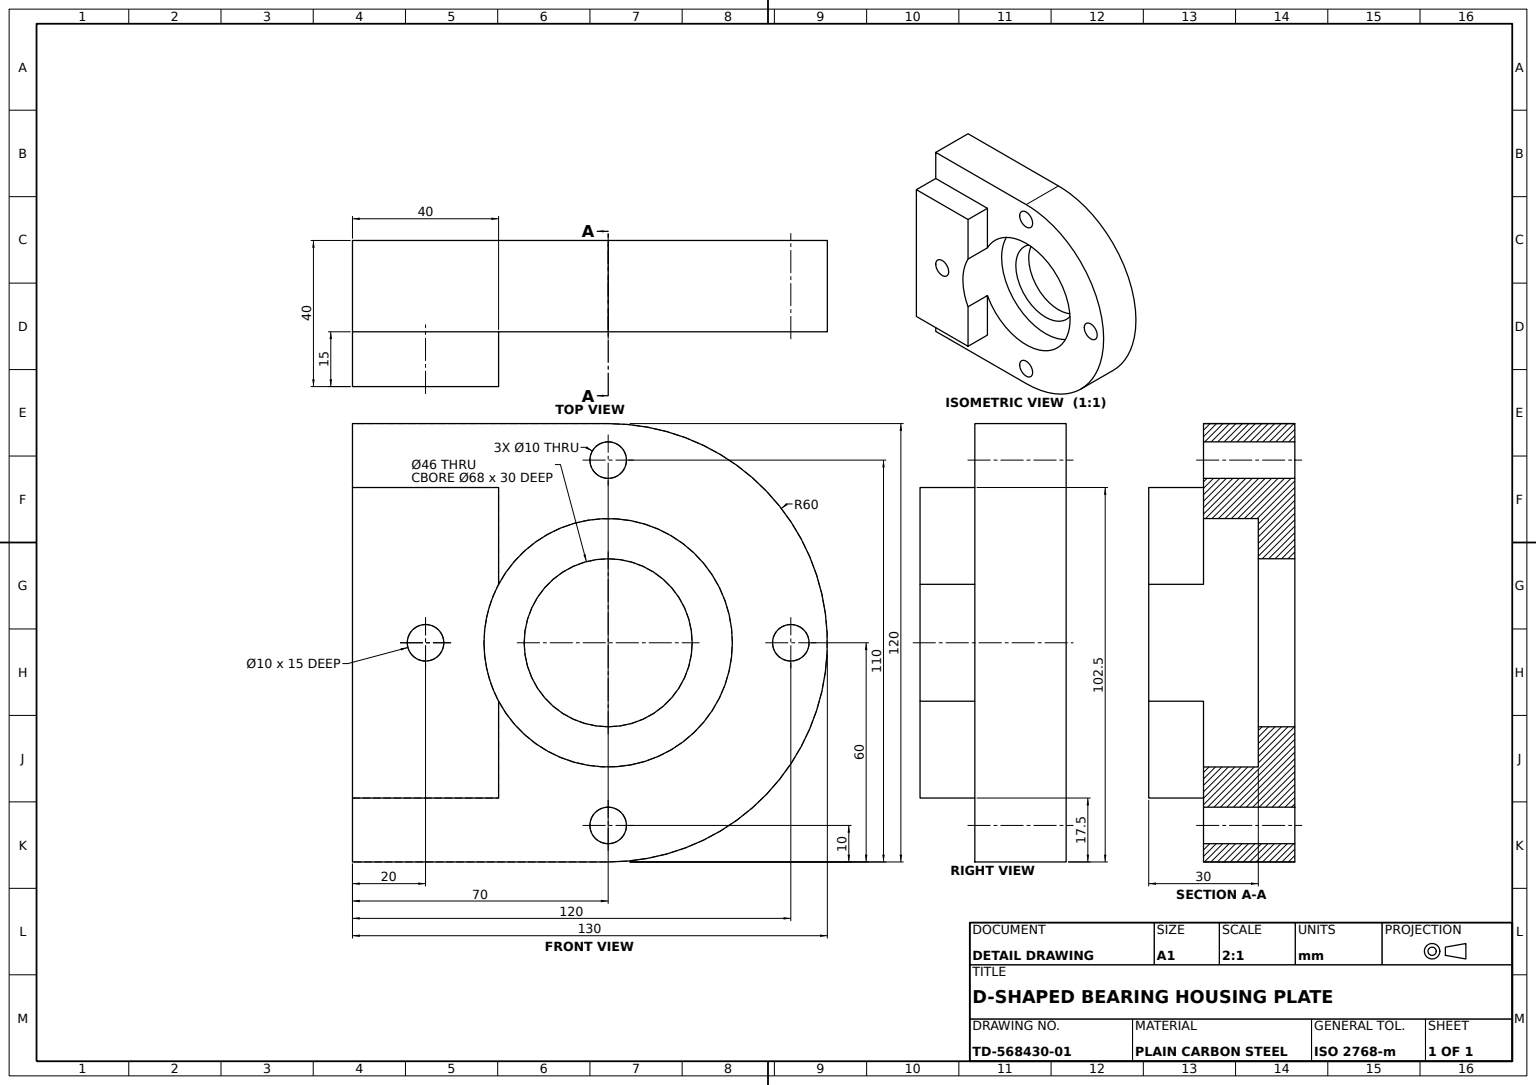
SolidWorks part; units mm, degrees
material "Plain Carbon Steel"
ref_plane "Front Plane" through (0, 0, 0) normal (0, 0, 1) x (1, 0, 0)
ref_plane "Top Plane" through (0, 0, 0) normal (0, 1, 0) x (1, 0, 0)
ref_plane "Right Plane" through (0, 0, 0) normal (1, 0, 0) x (0, 0, -1)
sketch "Base Plate Sketch" plane through (0, 0, 0) normal (0, 0, 1) x (1, 0, 0)
  line L0 (0, 0) -> (70, 0)
  line L2 (70, 120) -> (0, 120)
  line L3 (0, 120) -> (0, 0)
  arc A0 (70, 0) -> (70, 120) centre (70, 60) ccw
  dimension "D1" = 120
  dimension "D2" = 60
  dimension "D3" = 70
extrude "Base Plate" add sketch "Base Plate Sketch" along normal blind 25
sketch "Side Block Sketch" plane through (0, 0, 25) normal (0, 0, 1) x (1, 0, 0)
  line L0 (0, 0) -> (70, 0) construction
  line L1 (0, 120) -> (0, 0) construction
  line L2 (0, 102.5) -> (40, 102.5)
  line L3 (40, 102.5) -> (40, 17.5)
  line L4 (40, 17.5) -> (0, 17.5)
  line L5 (0, 17.5) -> (0, 102.5)
  dimension "D1" = 40
  dimension "D2" = 17.5
  dimension "D3" = 102.5
extrude "Side Block" add sketch "Side Block Sketch" along normal blind 15
sketch "Counterbore Ø68 Sketch" plane through (0, 0, 25) normal (0, 0, 1) x (1, 0, 0)
  circle A0 centre (70, 60) radius 34
  dimension "D1" = 68
  dimension "D2" = 68
extrude "Counterbore Ø68" cut sketch "Counterbore Ø68 Sketch" against normal blind 15
sketch "Block Relief Ø68 Sketch" plane through (0, 0, 40) normal (0, 0, 1) x (1, 0, 0)
  line L0 (40, 76) -> (40, 44)
  line L1 (0, 102.5) -> (0, 17.5) construction
  arc A0 (40, 76) -> (40, 44) centre (70, 60) ccw
  dimension "D1" = 68
  dimension "D2" = 34
  dimension "D3" = 40
extrude "Block Relief Ø68" cut sketch "Block Relief Ø68 Sketch" against normal blind 15
sketch "Bore Ø46 Sketch" plane through (0, 0, 10) normal (0, 0, 1) x (1, 0, 0)
  circle A0 centre (70, 60) radius 23
  dimension "D1" = 46
  dimension "D2" = 46
extrude "Bore Ø46" cut sketch "Bore Ø46 Sketch" against normal blind 15
sketch "Block Hole Ø10 Sketch" plane through (0, 0, 40) normal (0, 0, 1) x (1, 0, 0)
  line L0 (0, 102.5) -> (0, 17.5) construction
  line L1 (0, 17.5) -> (40, 17.5) construction
  circle A0 centre (20, 60) radius 5
  dimension "D1" = 10
  dimension "D4" = 10
  dimension "D2" = 20
  dimension "D3" = 42.5
extrude "Block Hole Ø10" cut sketch "Block Hole Ø10 Sketch" against normal blind 15
sketch "Mounting Holes Sketch" plane through (0, 0, 25) normal (0, 0, 1) x (1, 0, 0)
  line L0 (0, 17.5) -> (0, 0) construction
  line L1 (0, 0) -> (70, 0) construction
  circle A1 centre (70, 110) radius 5
  circle A2 centre (120, 60) radius 5
  circle A3 centre (70, 10) radius 5
  dimension "D1" = 10
  dimension "D2" = 10
  dimension "D3" = 10
  dimension "D4" = 10
  dimension "D5" = 70
  dimension "D6" = 120
  dimension "D7" = 10
  dimension "D8" = 60
  dimension "D9" = 110
extrude "Mounting Holes 3xØ10" cut sketch "Mounting Holes Sketch" against normal blind 25
